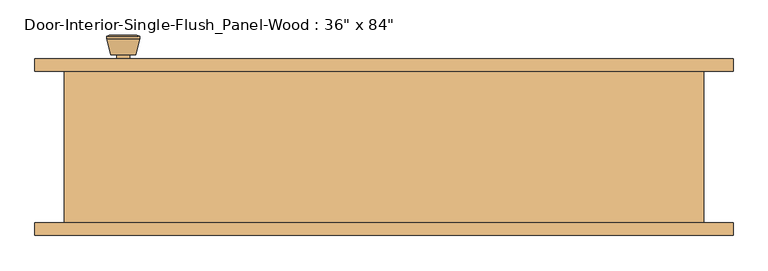
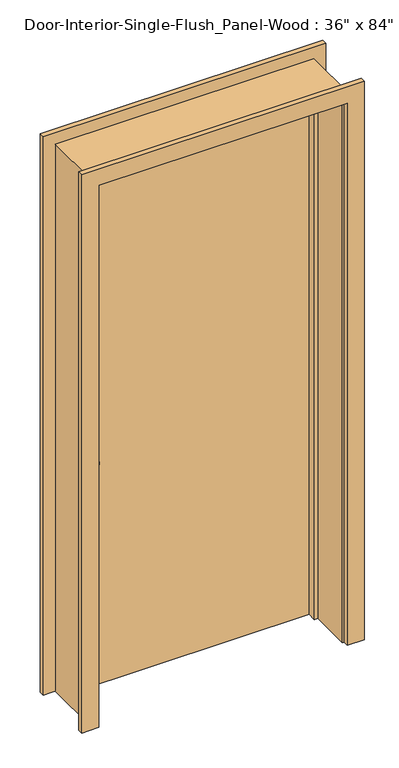
"""IFC4 building model written with IfcOpenShell, lengths in millimetres: door geometry."""

from ifc_helpers import new_model, si_unit, point, frame, frame_2d, origin, origin_with_axes, place, context, project, spatial, polyline, circle_curve, trimmed, segment, composite_curve, outline, extrude, faceted_brep, source, transform, mapped, element, save
from ifc_brep_helpers import plane_surface, cylinder_surface, revolved_surface, advanced_brep


def door_1d7b229f(model_context):
    return source(origin(), model_context, "Body", "SolidModel", [
        advanced_brep(
        [(-393.7, 70.2, 914.4), (-383.7, 70.2, 914.4), (-403.7, 70.2, 914.4), (-373.2241324, 21.2, 914.4), (-393.7, 21.2, 914.4), (-414.1758676, 21.2, 914.4), (-368.7, 23.0278681, 914.4), (-418.7, 23.0278681, 914.4), (-368.7, 26.4915463, 914.4), (-418.7, 26.4915463, 914.4), (-375.063764, 51.2, 914.4), (-412.336236, 51.2, 914.4), (-383.7, 51.2, 914.4), (-403.7, 51.2, 914.4)],
        [
            (0, 1),
            (1, 2, circle_curve(frame((-393.7, 70.2, 914.4), z_axis=(0.0, 1.0, 0.0), x_axis=(-1.0, 0.0, 0.0)), 10.0)),
            (2, 0),
            (2, 1, circle_curve(frame((-393.7, 70.2, 914.4), z_axis=(0.0, 1.0, 0.0), x_axis=(-1.0, 0.0, 0.0)), 10.0)),
            (3, 4),
            (4, 5),
            (5, 3, circle_curve(frame((-393.7, 21.2, 914.4), z_axis=(0.0, -1.0, 0.0), x_axis=(-1.0, 0.0, 0.0)), 20.4758676)),
            (3, 5, circle_curve(frame((-393.7, 21.2, 914.4), z_axis=(0.0, -1.0, 0.0), x_axis=(-1.0, 0.0, 0.0)), 20.4758676)),
            (6, 3),
            (5, 7),
            (7, 6, circle_curve(frame((-393.7, 23.0278681, 914.4), z_axis=(0.0, -1.0, 0.0), x_axis=(-1.0, 0.0, 0.0)), 25.0)),
            (6, 7, circle_curve(frame((-393.7, 23.0278681, 914.4), z_axis=(0.0, -1.0, 0.0), x_axis=(-1.0, 0.0, 0.0)), 25.0)),
            (8, 6),
            (7, 9),
            (9, 8, circle_curve(frame((-393.7, 26.4915463, 914.4), z_axis=(0.0, -1.0, 0.0), x_axis=(-1.0, 0.0, 0.0)), 25.0)),
            (8, 9, circle_curve(frame((-393.7, 26.4915463, 914.4), z_axis=(0.0, -1.0, 0.0), x_axis=(-1.0, 0.0, 0.0)), 25.0)),
            (10, 8),
            (9, 11),
            (11, 10, circle_curve(frame((-393.7, 51.2, 914.4), z_axis=(0.0, -1.0, 0.0), x_axis=(-1.0, 0.0, 0.0)), 18.636236)),
            (10, 11, circle_curve(frame((-393.7, 51.2, 914.4), z_axis=(0.0, -1.0, 0.0), x_axis=(-1.0, 0.0, 0.0)), 18.636236)),
            (12, 10),
            (11, 13),
            (13, 12, circle_curve(frame((-393.7, 51.2, 914.4), z_axis=(0.0, -1.0, 0.0), x_axis=(-1.0, 0.0, 0.0)), 10.0)),
            (12, 13, circle_curve(frame((-393.7, 51.2, 914.4), z_axis=(0.0, -1.0, 0.0), x_axis=(-1.0, 0.0, 0.0)), 10.0)),
            (1, 12),
            (13, 2),
        ],
        [
            plane_surface(frame((-393.7, 70.2, 914.4), z_axis=(0.0, 1.0, 0.0), x_axis=(-1.0, 0.0, 0.0))),
            plane_surface(frame((-393.7, 21.2, 914.4), z_axis=(0.0, -1.0, 0.0), x_axis=(-1.0, 0.0, 0.0))),
            revolved_surface(polyline([(-414.1758676, 21.2, 914.4), (-418.7, 23.0278681, 914.4)]), (-393.7, 70.2, 914.4), (0.0, 1.0, 0.0)),
            cylinder_surface(frame((-393.7, 70.2, 914.4), z_axis=(0.0, 1.0, 0.0), x_axis=(-1.0, 0.0, 0.0)), 25.0),
            revolved_surface(polyline([(-418.7, 26.4915463, 914.4), (-412.336236, 51.2, 914.4)]), (-393.7, 70.2, 914.4), (0.0, 1.0, 0.0)),
            plane_surface(frame((-393.7, 51.2, 914.4), z_axis=(0.0, 1.0, 0.0), x_axis=(-1.0, 0.0, 0.0))),
            cylinder_surface(frame((-393.7, 70.2, 914.4), z_axis=(0.0, 1.0, 0.0), x_axis=(-1.0, 0.0, 0.0)), 10.0),
        ],
        [
            (0, [[1, 2, 3]]),
            (0, [[-3, 4, -1]]),
            (1, [[5, 6, 7]]),
            (1, [[-6, -5, 8]]),
            (2, [[9, -7, 10, 11]]),
            (2, [[-10, -8, -9, 12]]),
            (3, [[13, -11, 14, 15]]),
            (3, [[-14, -12, -13, 16]]),
            (4, [[17, -15, 18, 19]]),
            (4, [[-18, -16, -17, 20]]),
            (5, [[21, -19, 22, 23]]),
            (5, [[-22, -20, -21, 24]]),
            (6, [[25, -23, 26, -2]]),
            (6, [[-26, -24, -25, -4]]),
        ],
    ),
        extrude(outline(composite_curve([segment(trimmed(circle_curve(frame_2d((914.4, -393.7)), 30.0), [point((914.4, -423.7))], [point((914.4, -363.7))], False, "CARTESIAN"), True, "CONTINUOUS"), segment(trimmed(circle_curve(frame_2d((914.4, -393.7)), 30.0), [point((914.4, -363.7))], [point((914.4, -423.7))], False, "CARTESIAN"), True, "CONTINUOUS")], self_intersect=False)), frame((0.0, 70.2, 0.0), z_axis=(0.0, 1.0, 0.0), x_axis=(0.0, 0.0, 1.0)), (0.0, 0.0, 1.0), 6.0),
        advanced_brep(
        [(-393.7, 117.125, 914.4), (-403.7, 117.125, 914.4), (-383.7, 117.125, 914.4), (-373.2241324, 166.125, 914.4), (-414.1758676, 166.125, 914.4), (-393.7, 166.125, 914.4), (-368.7, 164.2971319, 914.4), (-418.7, 164.2971319, 914.4), (-368.7, 160.8334537, 914.4), (-418.7, 160.8334537, 914.4), (-375.063764, 136.125, 914.4), (-412.336236, 136.125, 914.4), (-383.7, 136.125, 914.4), (-403.7, 136.125, 914.4)],
        [
            (0, 1),
            (1, 2, circle_curve(frame((-393.7, 117.125, 914.4), z_axis=(0.0, -1.0, 0.0), x_axis=(-1.0, 0.0, 0.0)), 10.0)),
            (2, 0),
            (2, 1, circle_curve(frame((-393.7, 117.125, 914.4), z_axis=(0.0, -1.0, 0.0), x_axis=(-1.0, 0.0, 0.0)), 10.0)),
            (3, 4, circle_curve(frame((-393.7, 166.125, 914.4), z_axis=(0.0, 1.0, 0.0), x_axis=(-1.0, 0.0, 0.0)), 20.4758676)),
            (4, 5),
            (5, 3),
            (4, 3, circle_curve(frame((-393.7, 166.125, 914.4), z_axis=(0.0, 1.0, 0.0), x_axis=(-1.0, 0.0, 0.0)), 20.4758676)),
            (6, 7, circle_curve(frame((-393.7, 164.2971319, 914.4), z_axis=(0.0, 1.0, 0.0), x_axis=(-1.0, 0.0, 0.0)), 25.0)),
            (7, 4),
            (3, 6),
            (7, 6, circle_curve(frame((-393.7, 164.2971319, 914.4), z_axis=(0.0, 1.0, 0.0), x_axis=(-1.0, 0.0, 0.0)), 25.0)),
            (8, 9, circle_curve(frame((-393.7, 160.8334537, 914.4), z_axis=(0.0, 1.0, 0.0), x_axis=(-1.0, 0.0, 0.0)), 25.0)),
            (9, 7),
            (6, 8),
            (9, 8, circle_curve(frame((-393.7, 160.8334537, 914.4), z_axis=(0.0, 1.0, 0.0), x_axis=(-1.0, 0.0, 0.0)), 25.0)),
            (10, 11, circle_curve(frame((-393.7, 136.125, 914.4), z_axis=(0.0, 1.0, 0.0), x_axis=(-1.0, 0.0, 0.0)), 18.636236)),
            (11, 9),
            (8, 10),
            (11, 10, circle_curve(frame((-393.7, 136.125, 914.4), z_axis=(0.0, 1.0, 0.0), x_axis=(-1.0, 0.0, 0.0)), 18.636236)),
            (12, 13, circle_curve(frame((-393.7, 136.125, 914.4), z_axis=(0.0, 1.0, 0.0), x_axis=(-1.0, 0.0, 0.0)), 10.0)),
            (13, 11),
            (10, 12),
            (13, 12, circle_curve(frame((-393.7, 136.125, 914.4), z_axis=(0.0, 1.0, 0.0), x_axis=(-1.0, 0.0, 0.0)), 10.0)),
            (1, 13),
            (12, 2),
        ],
        [
            plane_surface(frame((-393.7, 117.125, 914.4), z_axis=(0.0, -1.0, 0.0), x_axis=(-1.0, 0.0, 0.0))),
            plane_surface(frame((-393.7, 166.125, 914.4), z_axis=(0.0, 1.0, 0.0), x_axis=(-1.0, 0.0, 0.0))),
            revolved_surface(polyline([(-414.1758676, 166.125, 914.4), (-418.7, 164.2971319, 914.4)]), (-393.7, 117.125, 914.4), (0.0, -1.0, 0.0)),
            cylinder_surface(frame((-393.7, 117.125, 914.4), z_axis=(0.0, -1.0, 0.0), x_axis=(-1.0, 0.0, 0.0)), 25.0),
            revolved_surface(polyline([(-418.7, 160.8334537, 914.4), (-412.336236, 136.125, 914.4)]), (-393.7, 117.125, 914.4), (0.0, -1.0, 0.0)),
            plane_surface(frame((-393.7, 136.125, 914.4), z_axis=(0.0, -1.0, 0.0), x_axis=(-1.0, 0.0, 0.0))),
            cylinder_surface(frame((-393.7, 117.125, 914.4), z_axis=(0.0, -1.0, 0.0), x_axis=(-1.0, 0.0, 0.0)), 10.0),
        ],
        [
            (0, [[1, 2, 3]]),
            (0, [[-3, 4, -1]]),
            (1, [[5, 6, 7]]),
            (1, [[8, -7, -6]]),
            (2, [[9, 10, -5, 11]]),
            (2, [[12, -11, -8, -10]]),
            (3, [[13, 14, -9, 15]]),
            (3, [[16, -15, -12, -14]]),
            (4, [[17, 18, -13, 19]]),
            (4, [[20, -19, -16, -18]]),
            (5, [[21, 22, -17, 23]]),
            (5, [[24, -23, -20, -22]]),
            (6, [[-2, 25, -21, 26]]),
            (6, [[-4, -26, -24, -25]]),
        ],
    ),
        extrude(outline(composite_curve([segment(trimmed(circle_curve(frame_2d((914.4, -393.7)), 30.0), [point((914.4, -423.7))], [point((914.4, -363.7))], False, "CARTESIAN"), True, "CONTINUOUS"), segment(trimmed(circle_curve(frame_2d((914.4, -393.7)), 30.0), [point((914.4, -363.7))], [point((914.4, -423.7))], False, "CARTESIAN"), True, "CONTINUOUS")], self_intersect=False)), frame((0.0, 111.125, 0.0), z_axis=(0.0, 1.0, 0.0), x_axis=(0.0, 0.0, 1.0)), (0.0, 0.0, 1.0), 6.0),
        faceted_brep([(482.6, 111.125, 0.0), (482.6, -117.475, 0.0), (457.2, -117.475, 0.0), (457.2, 41.275, 0.0), (444.5, 41.275, 0.0), (444.5, 76.2, 0.0), (457.2, 76.2, 0.0), (457.2, 111.125, 0.0), (482.6, 111.125, 2159.0), (482.6, -117.475, 2159.0), (-482.6, -117.475, 2159.0), (-482.6, -117.475, 0.0), (-457.2, -117.475, 0.0), (-457.2, -117.475, 2133.6), (457.2, -117.475, 2133.6), (457.2, 41.275, 2133.6), (-457.2, 41.275, 2133.6), (-457.2, 41.275, 0.0), (-444.5, 41.275, 0.0), (-444.5, 41.275, 2120.9), (444.5, 41.275, 2120.9), (444.5, 76.2, 2120.9), (-444.5, 76.2, 2120.9), (-444.5, 76.2, 0.0), (-457.2, 76.2, 0.0), (-457.2, 76.2, 2133.6), (457.2, 76.2, 2133.6), (457.2, 111.125, 2133.6), (-457.2, 111.125, 2133.6), (-457.2, 111.125, 0.0), (-482.6, 111.125, 0.0), (-482.6, 111.125, 2159.0)], [[[0, 1, 2, 3, 4, 5, 6, 7]], [[1, 0, 8, 9]], [[2, 1, 9, 10, 11, 12, 13, 14]], [[3, 2, 14, 15]], [[4, 3, 15, 16, 17, 18, 19, 20]], [[5, 4, 20, 21]], [[6, 5, 21, 22, 23, 24, 25, 26]], [[7, 6, 26, 27]], [[0, 7, 27, 28, 29, 30, 31, 8]], [[9, 8, 31, 10]], [[15, 14, 13, 16]], [[21, 20, 19, 22]], [[27, 26, 25, 28]], [[30, 29, 24, 23, 18, 17, 12, 11]], [[10, 31, 30, 11]], [[16, 13, 12, 17]], [[22, 19, 18, 23]], [[28, 25, 24, 29]]]),
        extrude(outline(polyline([(457.2, 76.2), (-457.2, 76.2), (-457.2, 111.125), (457.2, 111.125), (457.2, 76.2)])), origin_with_axes(), (0.0, 0.0, 1.0), 2133.6),
        extrude(outline(polyline([(0.0, 463.55), (0.0, 527.05), (2203.45, 527.05), (2203.45, -527.05), (0.0, -527.05), (0.0, -463.55), (2139.95, -463.55), (2139.95, 463.55), (0.0, 463.55)])), frame((0.0, 111.125, 0.0), z_axis=(0.0, 1.0, 0.0), x_axis=(0.0, 0.0, 1.0)), (0.0, 0.0, 1.0), 19.05),
        extrude(outline(polyline([(0.0, 463.55), (0.0, 527.05), (2203.45, 527.05), (2203.45, -527.05), (0.0, -527.05), (0.0, -463.55), (2139.95, -463.55), (2139.95, 463.55), (0.0, 463.55)])), frame((0.0, -136.525, 0.0), z_axis=(0.0, 1.0, 0.0), x_axis=(0.0, 0.0, 1.0)), (0.0, 0.0, 1.0), 19.05),
    ])


if __name__ == "__main__":
    model = new_model("IFC4")
    model_context = context("Model", 3, world=origin())
    ifc_project = project(units=[si_unit("LENGTHUNIT", "METRE", prefix="MILLI")], contexts=[model_context])
    site = spatial("IfcSite", under=ifc_project)
    building = spatial("IfcBuilding", under=site)
    placement = place(None, origin())
    door_shape = door_1d7b229f(model_context)
    element("IfcDoor", 1, ObjectType="Door-Interior-Single-Flush_Panel-Wood : 36\" x 84\"", at=placement, inside=building, context=model_context, shape_type="MappedRepresentation", body=[
        mapped(door_shape, transform((0.0, 0.0, 0.0), x_axis=(1.0, 0.0, 0.0), y_axis=(0.0, 1.0, 0.0), z_axis=(0.0, 0.0, 1.0))),
    ])
    save(model, "model.ifc")

# Revit data of these elements
# Type "Door-Interior-Single-Flush_Panel-Wood : 36\" x 84\""
#   Type Mark = "8"
#   Assembly Code = "C1020300"
#   Analytic Construction = "Wooden"
#   Thickness = 0' - 1 3/8"
#   Thermal Resistance (R) = 2.5876 (h·ft²·°F)/BTU
#   Swing Angle [instance default] = 90.00°
#   Rough Width = 3' - 2"
#   Rough Height = 7' - 1"
#   Height = 7' - 0"
#   Width = 3' - 0"
#   Heat Transfer Coefficient (U) = 0.3865 BTU/(h·ft²·°F)
#   Trim Material = Cherry
#   Panel Material = Cherry
#   Frame Material = Cherry
#   Door Handle Material = Aluminum
#   Visual Light Transmittance = 0
#   Solar Heat Gain Coefficient = 0
#   Wall Closure = (empty or 0)
#   Function = (empty or 0)
# Element 1 (IfcDoor, "Door-Interior-Single-Flush_Panel-Wood : 36\" x 84\"")
#   Materials on its faces: "Cherry", "Aluminum"
# Materials
#   "Cherry": class "Wood", colour RGB 226 177 128, transparency 0, Description = "Prunus Serotina", Cost = 0
#   "Aluminum": class "Metal", colour RGB 247 247 247, transparency 0, Description = "Aluminum 6061", Cost = 0
